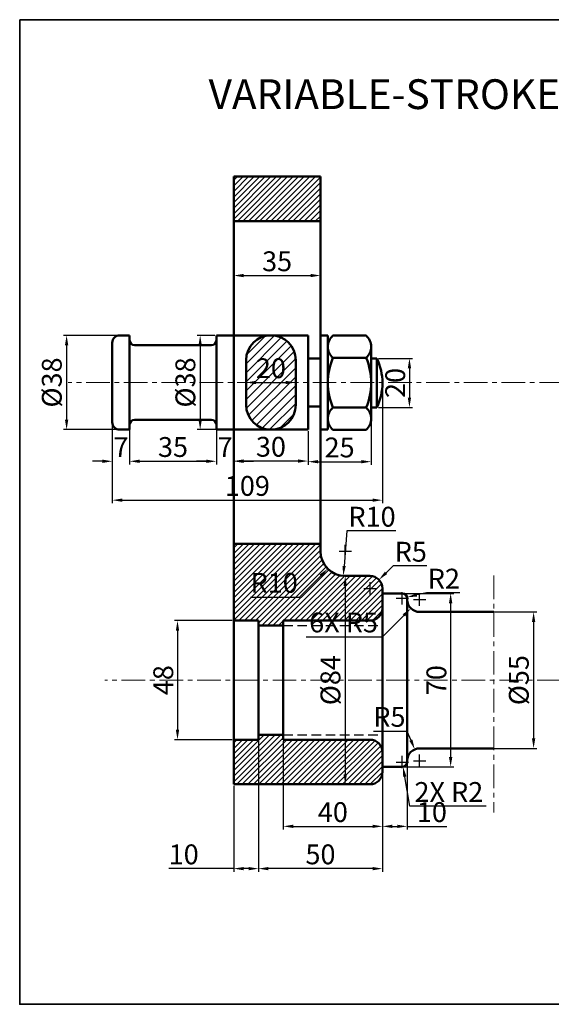
# Model space of a CAD drawing. Units: millimetres. Extents: x -135 to 382, y -21 to 376.
# Tile 1 of 2: x -135 to 80, y -21 to 376. Entities that reach past the tile are written whole.
import ezdxf

# ---------------------------------------------------------------- set-up
doc = ezdxf.new("R2010")
doc.units = ezdxf.units.MM
doc.header["$LTSCALE"] = 0.3
doc.linetypes.add('CENTER', pattern=[50.8, 31.75, -6.35, 6.35, -6.35])
doc.linetypes.add('DASHED', pattern=[19.05, 12.7, -6.35])
for name, color, linetype, lineweight in [('M-CNTR', 1, 'CENTER', 18), ('M-DIMS', 2, 'Continuous', 25), ('M-HATC', 8, 'Continuous', 18), ('M-HIDN', 6, 'DASHED', 25), ('M-OUTL', 7, 'Continuous', 50), ('M-TEXT', 3, 'Continuous', 25), ('M-TTLB', 7, 'Continuous', 35)]:
    doc.layers.add(name, color=color, linetype=linetype, lineweight=lineweight)
doc.styles.get("Standard").update_dxf_attribs({"font": 'arial.ttf'})
doc.dimstyles.new('ISO-25', dxfattribs={"dimtxt": 8, "dimasz": 4, "dimexe": 1.25, "dimexo": 0.625, "dimtad": 1, "dimtoh": 1, "dimdec": 0, "dimtxsty": 'Standard', "dimcen": 2.5, "dimadec": 0, "dimazin": 0, "dimtfac": 1, "dimtdec": 0, "dimtofl": 0, "dimtmove": 0, "dimatfit": 3, "dimfxl": 1, "dimarcsym": 0})

# ---------------------------------------------------------------- blocks, each defined once
blk = doc.blocks.new('*D1')
at = {"layer": 'Defpoints', "color": 0, "ltscale": 0.3, "transparency": 16777216}
for p in [(-48.44, 133.27), (-71.12, 85.27), (-48.44, 85.27)]:
    blk.add_point(p, dxfattribs=at)
at = {"layer": 'M-DIMS', "color": 0, "lineweight": -2, "ltscale": 0.3, "transparency": 16777216}
for p, q in [((-49.07, 133.27), (-72.37, 133.27)), ((-71.12, 129.27), (-71.12, 89.27)), ((-49.07, 85.27), (-72.37, 85.27))]:
    blk.add_line(p, q, dxfattribs=at)
at = {"layer": 'M-DIMS', "color": 0, "ltscale": 0.3, "transparency": 16777216}
for points in [[(-71.79, 129.27), (-70.46, 129.27), (-71.12, 133.27)], [(-71.79, 89.27), (-70.46, 89.27), (-71.12, 85.27)]]:
    blk.add_solid(points, dxfattribs=at)
at = {"layer": 'M-DIMS', "color": 0, "ltscale": 0.3, "transparency": 16777216, "insert": (-75.83, 109.27), "char_height": 8, "attachment_point": 5, "rotation": 90}
blk.add_mtext('48', dxfattribs=at)
blk = doc.blocks.new('*D2')
at = {"layer": 'Defpoints', "color": 0, "ltscale": 0.3, "transparency": 16777216}
for p in [(-3.44, 151.27), (-3.44, 67.27), (-3.44, 67.27)]:
    blk.add_point(p, dxfattribs=at)
at = {"layer": 'M-DIMS', "color": 0, "lineweight": -2, "ltscale": 0.3, "transparency": 16777216}
for p, q in [((-4.07, 151.27), (-4.69, 151.27)), ((-3.44, 147.27), (-3.44, 71.27)), ((-4.07, 67.27), (-4.69, 67.27))]:
    blk.add_line(p, q, dxfattribs=at)
at = {"layer": 'M-DIMS', "color": 0, "ltscale": 0.3, "transparency": 16777216}
for points in [[(-4.11, 147.27), (-2.78, 147.27), (-3.44, 151.27)], [(-4.11, 71.27), (-2.78, 71.27), (-3.44, 67.27)]]:
    blk.add_solid(points, dxfattribs=at)
at = {"layer": 'M-DIMS', "color": 0, "ltscale": 0.3, "transparency": 16777216, "insert": (-8.38, 109.27), "char_height": 8, "attachment_point": 5, "rotation": 90}
blk.add_mtext('%%C84', dxfattribs=at)
blk = doc.blocks.new('*D3')
at = {"layer": 'Defpoints', "color": 0, "ltscale": 0.3, "transparency": 16777216}
for p in [(15.56, 144.27), (15.56, 74.27), (39.08, 74.27)]:
    blk.add_point(p, dxfattribs=at)
at = {"layer": 'M-DIMS', "color": 0, "lineweight": -2, "ltscale": 0.3, "transparency": 16777216}
for p, q in [((16.18, 144.27), (40.33, 144.27)), ((39.08, 140.27), (39.08, 78.27)), ((16.18, 74.27), (40.33, 74.27))]:
    blk.add_line(p, q, dxfattribs=at)
at = {"layer": 'M-DIMS', "color": 0, "ltscale": 0.3, "transparency": 16777216}
for points in [[(38.41, 140.27), (39.75, 140.27), (39.08, 144.27)], [(38.41, 78.27), (39.75, 78.27), (39.08, 74.27)]]:
    blk.add_solid(points, dxfattribs=at)
at = {"layer": 'M-DIMS', "color": 0, "ltscale": 0.3, "transparency": 16777216, "insert": (34.37, 109.27), "char_height": 8, "attachment_point": 5, "rotation": 90}
blk.add_mtext('70', dxfattribs=at)
blk = doc.blocks.new('*D4')
at = {"layer": 'Defpoints', "color": 0, "ltscale": 0.3, "transparency": 16777216}
for p in [(49.48, 136.77), (49.48, 81.77), (72.56, 81.77)]:
    blk.add_point(p, dxfattribs=at)
at = {"layer": 'M-DIMS', "color": 0, "lineweight": -2, "ltscale": 0.3, "transparency": 16777216}
for p, q in [((50.1, 136.77), (73.81, 136.77)), ((72.56, 132.77), (72.56, 85.77)), ((50.1, 81.77), (73.81, 81.77))]:
    blk.add_line(p, q, dxfattribs=at)
at = {"layer": 'M-DIMS', "color": 0, "ltscale": 0.3, "transparency": 16777216}
for points in [[(71.89, 132.77), (73.22, 132.77), (72.56, 136.77)], [(71.89, 85.77), (73.22, 85.77), (72.56, 81.77)]]:
    blk.add_solid(points, dxfattribs=at)
at = {"layer": 'M-DIMS', "color": 0, "ltscale": 0.3, "transparency": 16777216, "insert": (67.62, 109.27), "char_height": 8, "attachment_point": 5, "rotation": 90}
blk.add_mtext('%%C55', dxfattribs=at)
blk = doc.blocks.new('*D5')
at = {"layer": 'Defpoints', "color": 0, "ltscale": 0.3, "transparency": 16777216}
for p in [(-38.44, 85.27), (-48.44, 67.27), (-38.44, 33.29)]:
    blk.add_point(p, dxfattribs=at)
at = {"layer": 'M-DIMS', "color": 0, "lineweight": -2, "ltscale": 0.3, "transparency": 16777216}
for p, q in [((-38.44, 84.64), (-38.44, 32.04)), ((-48.44, 66.64), (-48.44, 32.04)), ((-48.44, 33.29), (-74.58, 33.29)), ((-42.44, 33.29), (-44.44, 33.29))]:
    blk.add_line(p, q, dxfattribs=at)
at = {"layer": 'M-DIMS', "color": 0, "ltscale": 0.3, "transparency": 16777216}
for points in [[(-44.44, 33.95), (-44.44, 32.62), (-48.44, 33.29)], [(-42.44, 33.95), (-42.44, 32.62), (-38.44, 33.29)]]:
    blk.add_solid(points, dxfattribs=at)
at = {"layer": 'M-DIMS', "color": 0, "ltscale": 0.3, "transparency": 16777216, "insert": (-68.62, 38), "char_height": 8, "attachment_point": 5}
blk.add_mtext('10', dxfattribs=at)
blk = doc.blocks.new('*D6')
at = {"layer": 'Defpoints', "color": 0, "ltscale": 0.3, "transparency": 16777216}
for p in [(11.56, 74.27), (-38.44, 63.99), (-38.44, 33.29)]:
    blk.add_point(p, dxfattribs=at)
at = {"layer": 'M-DIMS', "color": 0, "lineweight": -2, "ltscale": 0.3, "transparency": 16777216}
for p, q in [((11.56, 73.64), (11.56, 32.04)), ((-38.44, 63.36), (-38.44, 32.04)), ((7.56, 33.29), (-34.44, 33.29))]:
    blk.add_line(p, q, dxfattribs=at)
at = {"layer": 'M-DIMS', "color": 0, "ltscale": 0.3, "transparency": 16777216}
for points in [[(-34.44, 33.95), (-34.44, 32.62), (-38.44, 33.29)], [(7.56, 33.95), (7.56, 32.62), (11.56, 33.29)]]:
    blk.add_solid(points, dxfattribs=at)
at = {"layer": 'M-DIMS', "color": 0, "ltscale": 0.3, "transparency": 16777216, "insert": (-13.44, 38), "char_height": 8, "attachment_point": 5}
blk.add_mtext('50', dxfattribs=at)
blk = doc.blocks.new('*D7')
at = {"layer": 'Defpoints', "color": 0, "ltscale": 0.3, "transparency": 16777216}
for p in [(-28.44, 85.27), (11.56, 85.27), (11.56, 50.33)]:
    blk.add_point(p, dxfattribs=at)
at = {"layer": 'M-DIMS', "color": 0, "lineweight": -2, "ltscale": 0.3, "transparency": 16777216}
for p, q in [((-28.44, 84.64), (-28.44, 49.08)), ((11.56, 84.64), (11.56, 49.08)), ((-24.44, 50.33), (7.56, 50.33))]:
    blk.add_line(p, q, dxfattribs=at)
at = {"layer": 'M-DIMS', "color": 0, "ltscale": 0.3, "transparency": 16777216}
for points in [[(-24.44, 51), (-24.44, 49.67), (-28.44, 50.33)], [(7.56, 51), (7.56, 49.67), (11.56, 50.33)]]:
    blk.add_solid(points, dxfattribs=at)
at = {"layer": 'M-DIMS', "color": 0, "ltscale": 0.3, "transparency": 16777216, "insert": (-8.44, 55.04), "char_height": 8, "attachment_point": 5}
blk.add_mtext('40', dxfattribs=at)
blk = doc.blocks.new('*D8')
at = {"layer": 'Defpoints', "color": 0, "ltscale": 0.3, "transparency": 16777216}
for p in [(11.56, 80.27), (21.56, 80.27), (21.56, 50.33)]:
    blk.add_point(p, dxfattribs=at)
at = {"layer": 'M-DIMS', "color": 0, "lineweight": -2, "ltscale": 0.3, "transparency": 16777216}
for p, q in [((11.56, 79.64), (11.56, 49.08)), ((21.56, 79.64), (21.56, 49.08)), ((15.56, 50.33), (17.56, 50.33)), ((21.56, 50.33), (37.49, 50.33))]:
    blk.add_line(p, q, dxfattribs=at)
at = {"layer": 'M-DIMS', "color": 0, "ltscale": 0.3, "transparency": 16777216}
for points in [[(15.56, 51), (15.56, 49.67), (11.56, 50.33)], [(17.56, 51), (17.56, 49.67), (21.56, 50.33)]]:
    blk.add_solid(points, dxfattribs=at)
at = {"layer": 'M-DIMS', "color": 0, "ltscale": 0.3, "transparency": 16777216, "insert": (31.52, 55.04), "char_height": 8, "attachment_point": 5}
blk.add_mtext('10', dxfattribs=at)
blk = doc.blocks.new('*D9')
at = {"layer": 'Defpoints', "color": 0, "ltscale": 0.3, "transparency": 16777216}
for p in [(-3.44, 161.27), (-4.22, 151.3)]:
    blk.add_point(p, dxfattribs=at)
at = {"layer": 'M-DIMS', "color": 0, "lineweight": -2, "ltscale": 0.3, "transparency": 16777216}
for p, q in [((-2.81, 169.41), (-3.91, 155.28)), ((16.91, 169.41), (-2.81, 169.41))]:
    blk.add_line(p, q, dxfattribs=at)
at = {"layer": 'M-DIMS', "color": 0, "ltscale": 0.3, "transparency": 16777216}
blk.add_solid([(-4.57, 155.34), (-3.25, 155.23), (-4.22, 151.3)], dxfattribs=at)
at = {"layer": 'M-DIMS', "color": 0, "ltscale": 0.3, "transparency": 16777216, "insert": (7.36, 174.12), "char_height": 8, "attachment_point": 5}
blk.add_mtext('R10', dxfattribs=at)
blk = doc.blocks.new('*D10')
at = {"layer": 'Defpoints', "color": 0, "ltscale": 0.3, "transparency": 16777216}
for p in [(10.15, 149.75), (6.56, 146.27)]:
    blk.add_point(p, dxfattribs=at)
at = {"layer": 'M-DIMS', "color": 0, "lineweight": -2, "ltscale": 0.3, "transparency": 16777216}
for p, q in [((15.9, 155.31), (13.02, 152.53)), ((29.48, 155.31), (15.9, 155.31)), ((6.56, 143.77), (6.56, 148.77)), ((4.06, 146.27), (9.06, 146.27))]:
    blk.add_line(p, q, dxfattribs=at)
at = {"layer": 'M-DIMS', "color": 0, "ltscale": 0.3, "transparency": 16777216}
blk.add_solid([(12.56, 153.01), (13.49, 152.05), (10.15, 149.75)], dxfattribs=at)
at = {"layer": 'M-DIMS', "color": 0, "ltscale": 0.3, "transparency": 16777216, "insert": (23, 160), "char_height": 8, "attachment_point": 5}
blk.add_mtext('R5', dxfattribs=at)
blk = doc.blocks.new('*D11')
at = {"layer": 'Defpoints', "color": 0, "ltscale": 0.3, "transparency": 16777216}
for p in [(19.56, 142.27), (21.51, 142.71)]:
    blk.add_point(p, dxfattribs=at)
at = {"layer": 'M-DIMS', "color": 0, "lineweight": -2, "ltscale": 0.3, "transparency": 16777216}
for p, q in [((19.56, 139.77), (19.56, 144.77)), ((29.3, 144.51), (25.4, 143.61)), ((42.75, 144.51), (29.3, 144.51)), ((17.06, 142.27), (22.06, 142.27))]:
    blk.add_line(p, q, dxfattribs=at)
at = {"layer": 'M-DIMS', "color": 0, "ltscale": 0.3, "transparency": 16777216}
blk.add_solid([(25.25, 144.26), (25.55, 142.96), (21.51, 142.71)], dxfattribs=at)
at = {"layer": 'M-DIMS', "color": 0, "ltscale": 0.3, "transparency": 16777216, "insert": (36.34, 149.15), "char_height": 8, "attachment_point": 5}
blk.add_mtext('R2', dxfattribs=at)
blk = doc.blocks.new('*D12')
at = {"layer": 'Defpoints', "color": 0, "ltscale": 0.3, "transparency": 16777216}
for p in [(24.6, 81.37), (26.56, 76.77)]:
    blk.add_point(p, dxfattribs=at)
at = {"layer": 'M-DIMS', "color": 0, "lineweight": -2, "ltscale": 0.3, "transparency": 16777216}
for p, q in [((7.89, 88.73), (21.47, 88.73)), ((21.47, 88.73), (23.04, 85.05)), ((24.06, 76.77), (29.06, 76.77)), ((26.56, 74.27), (26.56, 79.27))]:
    blk.add_line(p, q, dxfattribs=at)
at = {"layer": 'M-DIMS', "color": 0, "ltscale": 0.3, "transparency": 16777216}
blk.add_solid([(23.65, 85.31), (22.42, 84.79), (24.6, 81.37)], dxfattribs=at)
at = {"layer": 'M-DIMS', "color": 0, "ltscale": 0.3, "transparency": 16777216, "insert": (14.37, 93.43), "char_height": 8, "attachment_point": 5}
blk.add_mtext('R5', dxfattribs=at)
blk = doc.blocks.new('*D13')
at = {"layer": 'Defpoints', "color": 0, "ltscale": 0.3, "transparency": 16777216}
for p in [(-92.44, 248.27), (-115.87, 210.27), (-92.44, 210.27)]:
    blk.add_point(p, dxfattribs=at)
at = {"layer": 'M-DIMS', "color": 0, "lineweight": -2, "ltscale": 0.3, "transparency": 16777216}
for p, q in [((-93.07, 248.27), (-117.12, 248.27)), ((-115.87, 244.27), (-115.87, 214.27)), ((-93.07, 210.27), (-117.12, 210.27))]:
    blk.add_line(p, q, dxfattribs=at)
at = {"layer": 'M-DIMS', "color": 0, "ltscale": 0.3, "transparency": 16777216}
for points in [[(-116.54, 244.27), (-115.2, 244.27), (-115.87, 248.27)], [(-116.54, 214.27), (-115.2, 214.27), (-115.87, 210.27)]]:
    blk.add_solid(points, dxfattribs=at)
at = {"layer": 'M-DIMS', "color": 0, "ltscale": 0.3, "transparency": 16777216, "insert": (-120.8, 229.27), "char_height": 8, "attachment_point": 5, "rotation": 90}
blk.add_mtext('%%C38', dxfattribs=at)
blk = doc.blocks.new('*D14')
at = {"layer": 'Defpoints', "color": 0, "ltscale": 0.3, "transparency": 16777216}
for p in [(-97.44, 219.54), (-90.44, 219.54), (-90.44, 197.51)]:
    blk.add_point(p, dxfattribs=at)
at = {"layer": 'M-DIMS', "color": 0, "lineweight": -2, "ltscale": 0.3, "transparency": 16777216}
for p, q in [((-97.44, 218.92), (-97.44, 196.26)), ((-90.44, 218.92), (-90.44, 196.26)), ((-101.44, 197.51), (-105.44, 197.51)), ((-86.44, 197.51), (-82.44, 197.51))]:
    blk.add_line(p, q, dxfattribs=at)
at = {"layer": 'M-DIMS', "color": 0, "ltscale": 0.3, "transparency": 16777216}
for points in [[(-101.44, 198.17), (-101.44, 196.84), (-97.44, 197.51)], [(-86.44, 198.17), (-86.44, 196.84), (-90.44, 197.51)]]:
    blk.add_solid(points, dxfattribs=at)
at = {"layer": 'M-DIMS', "color": 0, "ltscale": 0.3, "transparency": 16777216, "insert": (-93.94, 202.13), "char_height": 8, "attachment_point": 5}
blk.add_mtext('7', dxfattribs=at)
blk = doc.blocks.new('*D15')
at = {"layer": 'Defpoints', "color": 0, "ltscale": 0.3, "transparency": 16777216}
for p in [(-90.44, 222.54), (-55.44, 222.54), (-55.44, 197.51)]:
    blk.add_point(p, dxfattribs=at)
at = {"layer": 'M-DIMS', "color": 0, "lineweight": -2, "ltscale": 0.3, "transparency": 16777216}
for p, q in [((-90.44, 221.92), (-90.44, 196.26)), ((-55.44, 221.92), (-55.44, 196.26)), ((-86.44, 197.51), (-59.44, 197.51))]:
    blk.add_line(p, q, dxfattribs=at)
at = {"layer": 'M-DIMS', "color": 0, "ltscale": 0.3, "transparency": 16777216}
for points in [[(-86.44, 198.17), (-86.44, 196.84), (-90.44, 197.51)], [(-59.44, 198.17), (-59.44, 196.84), (-55.44, 197.51)]]:
    blk.add_solid(points, dxfattribs=at)
at = {"layer": 'M-DIMS', "color": 0, "ltscale": 0.3, "transparency": 16777216, "insert": (-72.94, 202.22), "char_height": 8, "attachment_point": 5}
blk.add_mtext('35', dxfattribs=at)
blk = doc.blocks.new('*D16')
at = {"layer": 'Defpoints', "color": 0, "ltscale": 0.3, "transparency": 16777216}
for p in [(-55.44, 222.54), (-48.44, 218.5), (-48.44, 197.51)]:
    blk.add_point(p, dxfattribs=at)
at = {"layer": 'M-DIMS', "color": 0, "lineweight": -2, "ltscale": 0.3, "transparency": 16777216}
for p, q in [((-55.44, 221.92), (-55.44, 196.26)), ((-48.44, 217.88), (-48.44, 196.26)), ((-59.44, 197.51), (-63.44, 197.51)), ((-44.44, 197.51), (-40.44, 197.51))]:
    blk.add_line(p, q, dxfattribs=at)
at = {"layer": 'M-DIMS', "color": 0, "ltscale": 0.3, "transparency": 16777216}
for points in [[(-59.44, 198.17), (-59.44, 196.84), (-55.44, 197.51)], [(-44.44, 198.17), (-44.44, 196.84), (-48.44, 197.51)]]:
    blk.add_solid(points, dxfattribs=at)
at = {"layer": 'M-DIMS', "color": 0, "ltscale": 0.3, "transparency": 16777216, "insert": (-51.94, 202.13), "char_height": 8, "attachment_point": 5}
blk.add_mtext('7', dxfattribs=at)
blk = doc.blocks.new('*D17')
at = {"layer": 'Defpoints', "color": 0, "ltscale": 0.3, "transparency": 16777216}
for p in [(-18.44, 210.27), (-48.44, 201.14), (-48.44, 197.6)]:
    blk.add_point(p, dxfattribs=at)
at = {"layer": 'M-DIMS', "color": 0, "lineweight": -2, "ltscale": 0.3, "transparency": 16777216}
for p, q in [((-18.44, 209.64), (-18.44, 196.35)), ((-48.44, 200.52), (-48.44, 196.35)), ((-22.44, 197.6), (-44.44, 197.6))]:
    blk.add_line(p, q, dxfattribs=at)
at = {"layer": 'M-DIMS', "color": 0, "ltscale": 0.3, "transparency": 16777216}
for points in [[(-44.44, 198.27), (-44.44, 196.94), (-48.44, 197.6)], [(-22.44, 198.27), (-22.44, 196.94), (-18.44, 197.6)]]:
    blk.add_solid(points, dxfattribs=at)
at = {"layer": 'M-DIMS', "color": 0, "ltscale": 0.3, "transparency": 16777216, "insert": (-33.44, 202.32), "char_height": 8, "attachment_point": 5}
blk.add_mtext('30', dxfattribs=at)
blk = doc.blocks.new('*D18')
at = {"layer": 'Defpoints', "color": 0, "ltscale": 0.3, "transparency": 16777216}
for p in [(-97.44, 229.27), (11.56, 229.27), (11.56, 181.83)]:
    blk.add_point(p, dxfattribs=at)
at = {"layer": 'M-DIMS', "color": 0, "lineweight": -2, "ltscale": 0.3, "transparency": 16777216}
for p, q in [((-97.44, 228.64), (-97.44, 180.58)), ((11.56, 228.64), (11.56, 180.58)), ((-93.44, 181.83), (7.56, 181.83))]:
    blk.add_line(p, q, dxfattribs=at)
at = {"layer": 'M-DIMS', "color": 0, "ltscale": 0.3, "transparency": 16777216}
for points in [[(-93.44, 182.5), (-93.44, 181.17), (-97.44, 181.83)], [(7.56, 182.5), (7.56, 181.17), (11.56, 181.83)]]:
    blk.add_solid(points, dxfattribs=at)
at = {"layer": 'M-DIMS', "color": 0, "ltscale": 0.3, "transparency": 16777216, "insert": (-42.94, 186.54), "char_height": 8, "attachment_point": 5}
blk.add_mtext('109', dxfattribs=at)
blk = doc.blocks.new('*D19')
at = {"layer": 'Defpoints', "color": 0, "ltscale": 0.3, "transparency": 16777216}
for p in [(7.01, 214.74), (-18.44, 203), (7.01, 197.34)]:
    blk.add_point(p, dxfattribs=at)
at = {"layer": 'M-DIMS', "color": 0, "lineweight": -2, "ltscale": 0.3, "transparency": 16777216}
for p, q in [((7.01, 214.11), (7.01, 196.09)), ((-18.44, 202.37), (-18.44, 196.09)), ((-14.44, 197.34), (3.01, 197.34))]:
    blk.add_line(p, q, dxfattribs=at)
at = {"layer": 'M-DIMS', "color": 0, "ltscale": 0.3, "transparency": 16777216}
for points in [[(-14.44, 198.01), (-14.44, 196.68), (-18.44, 197.34)], [(3.01, 198.01), (3.01, 196.68), (7.01, 197.34)]]:
    blk.add_solid(points, dxfattribs=at)
at = {"layer": 'M-DIMS', "color": 0, "ltscale": 0.3, "transparency": 16777216, "insert": (-5.72, 202.05), "char_height": 8, "attachment_point": 5}
blk.add_mtext('25', dxfattribs=at)
blk = doc.blocks.new('*D20')
at = {"layer": 'Defpoints', "color": 0, "ltscale": 0.3, "transparency": 16777216}
for p in [(-13.44, 272.39), (-48.44, 268.37), (-13.44, 268.37)]:
    blk.add_point(p, dxfattribs=at)
at = {"layer": 'M-DIMS', "color": 0, "lineweight": -2, "ltscale": 0.3, "transparency": 16777216}
for p, q in [((-48.44, 269), (-48.44, 273.64)), ((-44.44, 272.39), (-17.44, 272.39)), ((-13.44, 269), (-13.44, 273.64))]:
    blk.add_line(p, q, dxfattribs=at)
at = {"layer": 'M-DIMS', "color": 0, "ltscale": 0.3, "transparency": 16777216}
for points in [[(-44.44, 273.05), (-44.44, 271.72), (-48.44, 272.39)], [(-17.44, 273.05), (-17.44, 271.72), (-13.44, 272.39)]]:
    blk.add_solid(points, dxfattribs=at)
at = {"layer": 'M-DIMS', "color": 0, "ltscale": 0.3, "transparency": 16777216, "insert": (-30.94, 277.1), "char_height": 8, "attachment_point": 5}
blk.add_mtext('35', dxfattribs=at)
blk = doc.blocks.new('*D21')
at = {"layer": 'Defpoints', "color": 0, "ltscale": 0.3, "transparency": 16777216}
for p in [(-55.44, 248.27), (-61.98, 210.27), (-54.29, 210.27)]:
    blk.add_point(p, dxfattribs=at)
at = {"layer": 'M-DIMS', "color": 0, "lineweight": -2, "ltscale": 0.3, "transparency": 16777216}
for p, q in [((-56.07, 248.27), (-63.23, 248.27)), ((-61.98, 244.27), (-61.98, 214.27)), ((-54.91, 210.27), (-63.23, 210.27))]:
    blk.add_line(p, q, dxfattribs=at)
at = {"layer": 'M-DIMS', "color": 0, "ltscale": 0.3, "transparency": 16777216}
for points in [[(-62.65, 244.27), (-61.31, 244.27), (-61.98, 248.27)], [(-62.65, 214.27), (-61.31, 214.27), (-61.98, 210.27)]]:
    blk.add_solid(points, dxfattribs=at)
at = {"layer": 'M-DIMS', "color": 0, "ltscale": 0.3, "transparency": 16777216, "insert": (-66.91, 229.27), "char_height": 8, "attachment_point": 5, "rotation": 90}
blk.add_mtext('%%C38', dxfattribs=at)
blk = doc.blocks.new('*D22')
at = {"layer": 'Defpoints', "color": 0, "ltscale": 0.3, "transparency": 16777216}
for p in [(9.28, 239), (9.28, 219.16), (22.45, 219.16)]:
    blk.add_point(p, dxfattribs=at)
at = {"layer": 'M-DIMS', "color": 0, "lineweight": -2, "ltscale": 0.3, "transparency": 16777216}
for p, q in [((9.91, 239), (23.7, 239)), ((22.45, 235), (22.45, 223.16)), ((9.91, 219.16), (23.7, 219.16))]:
    blk.add_line(p, q, dxfattribs=at)
at = {"layer": 'M-DIMS', "color": 0, "ltscale": 0.3, "transparency": 16777216}
for points in [[(21.79, 235), (23.12, 235), (22.45, 239)], [(21.79, 223.16), (23.12, 223.16), (22.45, 219.16)]]:
    blk.add_solid(points, dxfattribs=at)
at = {"layer": 'M-DIMS', "color": 0, "ltscale": 0.3, "transparency": 16777216, "insert": (17.75, 229.08), "char_height": 8, "attachment_point": 5, "rotation": 90}
blk.add_mtext('20', dxfattribs=at)
blk = doc.blocks.new('*D23')
at = {"layer": 'Defpoints', "color": 0, "ltscale": 0.3, "transparency": 16777216}
for p in [(-43.44, 229.27), (-23.44, 229.27), (-23.44, 229.27)]:
    blk.add_point(p, dxfattribs=at)
at = {"layer": 'M-DIMS', "color": 0, "lineweight": -2, "ltscale": 0.3, "transparency": 16777216}
for p, q in [((-43.44, 229.89), (-43.44, 230.52)), ((-23.44, 229.89), (-23.44, 230.52)), ((-39.44, 229.27), (-27.44, 229.27))]:
    blk.add_line(p, q, dxfattribs=at)
at = {"layer": 'M-DIMS', "color": 0, "ltscale": 0.3, "transparency": 16777216}
for points in [[(-39.44, 229.93), (-39.44, 228.6), (-43.44, 229.27)], [(-27.44, 229.93), (-27.44, 228.6), (-23.44, 229.27)]]:
    blk.add_solid(points, dxfattribs=at)
at = {"layer": 'M-DIMS', "color": 0, "ltscale": 0.3, "transparency": 16777216, "insert": (-33.44, 233.98), "char_height": 8, "attachment_point": 5}
blk.add_mtext('20', dxfattribs=at)
blk = doc.blocks.new('*D37')
at = {"layer": 'Defpoints', "color": 0, "ltscale": 0.3, "transparency": 16777216}
for p in [(-3.44, 161.27), (-10.51, 154.2)]:
    blk.add_point(p, dxfattribs=at)
at = {"layer": 'M-DIMS', "color": 0, "lineweight": -2, "ltscale": 0.3, "transparency": 16777216}
for p, q in [((-3.44, 158.77), (-3.44, 163.77)), ((-5.94, 161.27), (-0.94, 161.27)), ((-21.95, 142.76), (-13.34, 151.37)), ((-41.66, 142.76), (-21.95, 142.76))]:
    blk.add_line(p, q, dxfattribs=at)
at = {"layer": 'M-DIMS', "color": 0, "ltscale": 0.3, "transparency": 16777216}
blk.add_solid([(-13.81, 151.84), (-12.87, 150.9), (-10.51, 154.2)], dxfattribs=at)
at = {"layer": 'M-DIMS', "color": 0, "ltscale": 0.3, "transparency": 16777216, "insert": (-32.12, 147.47), "char_height": 8, "attachment_point": 5}
blk.add_mtext('R10', dxfattribs=at)
blk = doc.blocks.new('*D38')
at = {"layer": 'Defpoints', "color": 0, "ltscale": 0.3, "transparency": 16777216}
for p in [(26.56, 141.77), (23.03, 138.23)]:
    blk.add_point(p, dxfattribs=at)
at = {"layer": 'M-DIMS', "color": 0, "lineweight": -2, "ltscale": 0.3, "transparency": 16777216}
for p, q in [((26.56, 139.27), (26.56, 144.27)), ((24.06, 141.77), (29.06, 141.77)), ((11.61, 126.78), (20.2, 135.39)), ((-19.21, 126.78), (11.61, 126.78))]:
    blk.add_line(p, q, dxfattribs=at)
at = {"layer": 'M-DIMS', "color": 0, "ltscale": 0.3, "transparency": 16777216}
blk.add_solid([(19.73, 135.86), (20.67, 134.92), (23.03, 138.23)], dxfattribs=at)
at = {"layer": 'M-DIMS', "color": 0, "ltscale": 0.3, "transparency": 16777216, "insert": (-4.11, 131.49), "char_height": 8, "attachment_point": 5}
blk.add_mtext('6X R5', dxfattribs=at)
blk = doc.blocks.new('*D39')
at = {"layer": 'Defpoints', "color": 0, "ltscale": 0.3, "transparency": 16777216}
for p in [(19.56, 76.27), (19.9, 74.3)]:
    blk.add_point(p, dxfattribs=at)
at = {"layer": 'M-DIMS', "color": 0, "lineweight": -2, "ltscale": 0.3, "transparency": 16777216}
for p, q in [((17.06, 76.27), (22.06, 76.27)), ((19.56, 73.77), (19.56, 78.77)), ((22.66, 58.5), (20.59, 70.36)), ((53.43, 58.5), (22.66, 58.5))]:
    blk.add_line(p, q, dxfattribs=at)
at = {"layer": 'M-DIMS', "color": 0, "ltscale": 0.3, "transparency": 16777216}
blk.add_solid([(21.25, 70.47), (19.93, 70.24), (19.9, 74.3)], dxfattribs=at)
at = {"layer": 'M-DIMS', "color": 0, "ltscale": 0.3, "transparency": 16777216, "insert": (38.36, 63.14), "char_height": 8, "attachment_point": 5}
blk.add_mtext('2X R2', dxfattribs=at)

msp = doc.modelspace()

# ---------------------------------------------------------------- hatches: boundary and pattern name
at = {"layer": 'M-HATC', "ltscale": 0.3}
h = msp.add_hatch(dxfattribs=at)
h.set_pattern_fill('ANSI31', color=256, scale=0.5)
h.paths.add_polyline_path([(-13.44, 312.27), (-48.44, 312.27), (-48.44, 294.27), (-13.44, 294.27)])
h.paths.add_polyline_path([(11.56, 146.27, 0.414214), (6.56, 151.27), (-3.44, 151.27, -0.414214), (-13.44, 161.27), (-13.44, 164.27), (-48.44, 164.27), (-48.44, 133.27), (-38.44, 133.27), (-38.44, 131.27), (-28.44, 131.27), (-28.44, 133.27), (6.56, 133.27, 0.414214), (11.56, 138.27)])
h.paths.add_polyline_path([(11.56, 80.27, 0.414214), (6.56, 85.27), (-28.44, 85.27), (-28.44, 87.27), (-38.44, 87.27), (-38.44, 85.27), (-48.44, 85.27), (-48.44, 67.27), (6.56, 67.27, 0.414214), (11.56, 72.27)])
h = msp.add_hatch(dxfattribs=at)
h.set_pattern_fill('ANSI31', color=256, scale=0.8)
h.paths.add_polyline_path([(-23.44, 238.27, 1), (-43.44, 238.27), (-43.44, 229.27), (-23.44, 229.27)])
h.paths.add_polyline_path([(-23.44, 229.27), (-43.44, 229.27), (-43.44, 220.27, 1), (-23.44, 220.27)])

# ---------------------------------------------------------------- linework, layer by layer
at = {"layer": 'M-CNTR'}
for p, q in [((145.36, 229.27), (-115.25, 229.27)), ((56.56, 151.5), (56.56, 55.89)), ((266.38, 109.27), (-100.48, 109.27))]:
    msp.add_line(p, q, dxfattribs=at)
at = {"layer": 'M-HIDN'}
for p, q in [((-28.44, 131.27), (11.56, 131.27)), ((-28.44, 87.27), (11.56, 87.27))]:
    msp.add_line(p, q, dxfattribs=at)
at = {"layer": 'M-OUTL'}
for p, q in [((-48.44, 312.27), (-48.44, 67.27)), ((-48.44, 312.27), (-13.44, 312.27)), ((-13.44, 312.27), (-13.44, 161.27)), ((6.56, 151.27), (-3.44, 151.27)), ((11.56, 72.27), (11.56, 146.27)), ((11.56, 144.27), (19.56, 144.27)), ((21.56, 142.27), (21.56, 141.77)), ((21.56, 76.27), (21.56, 142.27)), ((26.56, 136.77), (56.56, 136.77)), ((-48.44, 133.27), (-48.44, 85.27)), ((-38.44, 133.27), (-48.44, 133.27)), ((-38.44, 85.27), (-38.44, 133.27)), ((-38.44, 131.27), (-38.44, 87.27)), ((-38.44, 131.27), (-28.44, 131.27)), ((6.56, 133.27), (-28.44, 133.27)), ((-28.44, 133.27), (-28.44, 85.27)), ((-28.44, 87.27), (-28.44, 131.27)), ((-48.44, 85.27), (-38.44, 85.27)), ((-38.44, 87.27), (-28.44, 87.27)), ((-28.44, 85.27), (6.56, 85.27)), ((56.56, 81.77), (26.56, 81.77)), ((21.56, 76.77), (21.56, 76.27)), ((19.56, 74.27), (11.56, 74.27)), ((-48.44, 67.27), (6.56, 67.27))]:
    msp.add_line(p, q, dxfattribs=at)
at = {"layer": 'M-OUTL', "ltscale": 0.3}
for p, q in [((-13.44, 294.27), (-48.44, 294.27)), ((-94.44, 248.27), (-90.44, 248.27)), ((-90.44, 248.27), (-90.44, 246.27)), ((-90.44, 246.27), (-90.44, 210.27)), ((-55.44, 246.27), (-55.44, 248.27)), ((-55.44, 248.27), (-48.44, 248.27)), ((-55.44, 246.27), (-55.44, 212.27)), ((-48.44, 248.27), (-48.44, 210.27)), ((-48.44, 248.27), (-18.44, 248.27)), ((-18.44, 248.27), (-18.44, 210.27)), ((-13.44, 248.27), (-10.44, 248.27)), ((-10.44, 248.27), (-10.44, 210.27)), ((-1.41, 248.16), (-8.44, 248.16)), ((5.01, 248.16), (-1.41, 248.16)), ((-97.44, 213.27), (-97.44, 245.27)), ((-88.44, 244.27), (-57.44, 244.27)), ((-10.44, 243.95), (-10.44, 214.59)), ((7.01, 214.59), (7.01, 243.95)), ((-43.44, 220.27), (-43.44, 238.27)), ((-23.44, 220.27), (-23.44, 238.27)), ((-13.44, 239), (-18.44, 239)), ((-8.44, 239.16), (-1.41, 239.16)), ((-1.41, 239.16), (5.01, 239.16)), ((7.01, 239), (9.28, 239)), ((9.28, 239), (9.28, 219.16)), ((11.56, 229.08), (11.56, 229.27)), ((-13.44, 219.54), (-18.44, 219.54)), ((-8.44, 219.16), (-1.41, 219.16)), ((-1.41, 219.16), (5.01, 219.16)), ((7.01, 219.16), (9.28, 219.16)), ((-57.44, 214.27), (-88.44, 214.27)), ((-55.44, 210.27), (-55.44, 212.27)), ((-90.44, 210.27), (-94.44, 210.27)), ((-48.44, 210.27), (-55.44, 210.27)), ((-18.44, 210.27), (-48.44, 210.27)), ((-10.44, 210.27), (-13.44, 210.27)), ((-8.44, 210.16), (-1.41, 210.16)), ((-1.41, 210.16), (5.01, 210.16)), ((-48.44, 164.27), (-13.44, 164.27))]:
    msp.add_line(p, q, dxfattribs=at)
for centre, radius, start, end in [((-94.44, 245.27), 3, 90, 180), ((-88.44, 246.27), 2, 180, 270), ((-57.44, 246.27), 2, 270, 0), ((-33.44, 238.27), 10, 0, 180), ((-4.4, 243.66), 6.05, 131.9333, 228.0667), ((0.97, 243.66), 6.05, 311.9333, 48.0667), ((15.56, 229.16), 26, 157.3801, 202.6199), ((-18.99, 229.16), 26, 337.3801, 22.6199), ((-11.2, 229.08), 22.76, 334.1686, 25.8314), ((-33.44, 220.27), 10, 180, 0), ((-4.38, 214.66), 6.06, 132.0649, 227.9351), ((0.95, 214.66), 6.06, 312.0649, 47.9351), ((-94.44, 213.27), 3, 180, 270), ((-88.44, 212.27), 2, 90, 180), ((-57.44, 212.27), 2, 0, 90)]:
    msp.add_arc(centre, radius, start, end, dxfattribs=at)
at = {"layer": 'M-OUTL'}
for centre, radius, start, end in [((-3.44, 161.27), 10, 180, 270), ((6.56, 146.27), 5, 0, 90), ((19.56, 142.27), 2, 0, 90), ((26.56, 141.77), 5, 180, 270), ((6.56, 138.27), 5, 270, 0), ((6.56, 80.27), 5, 0, 90), ((26.56, 76.77), 5, 90, 180), ((19.56, 76.27), 2, 270, 0), ((6.56, 72.27), 5, 270, 0)]:
    msp.add_arc(centre, radius, start, end, dxfattribs=at)
at = {"layer": 'M-TTLB', "ltscale": 0.3}
msp.add_lwpolyline([(-134.8, 375.53), (381.64, 375.53), (381.64, -21.41), (-134.8, -21.41)], close=True, dxfattribs=at)

# ---------------------------------------------------------------- texts
at = {"layer": 'M-TEXT', "ltscale": 0.3, "insert": (-77.37, 351.5), "char_height": 12, "attachment_point": 1}
msp.add_mtext_dynamic_manual_height_columns('\\pxqc;VARIABLE-STROKE CRANK LEVER', width=287.9223, gutter_width=12.5, heights=[0], dxfattribs=at)

# ---------------------------------------------------------------- dimensions: what is measured, and where the dimension line sits
at = {"layer": 'M-DIMS', "ltscale": 0.3}
for base, p1, p2, picture, middle in [((-13.44, 272.39), (-48.44, 268.37), (-13.44, 268.37), '*D20', (-30.94, 277.1)), ((-23.44, 229.27), (-43.44, 229.27), (-23.44, 229.27), '*D23', (-33.44, 233.98)), ((11.56, 181.83), (-97.44, 229.27), (11.56, 229.27), '*D18', (-42.94, 186.54)), ((-55.44, 197.51), (-90.44, 222.54), (-55.44, 222.54), '*D15', (-72.94, 202.22)), ((-48.44, 197.51), (-55.44, 222.54), (-48.44, 218.5), '*D16', (-51.94, 202.13)), ((-90.44, 197.51), (-97.44, 219.54), (-90.44, 219.54), '*D14', (-93.94, 202.13)), ((7.01, 197.34), (-18.44, 203), (7.01, 214.74), '*D19', (-5.72, 202.05)), ((-48.44, 197.6), (-18.44, 210.27), (-48.44, 201.14), '*D17', (-33.44, 202.32)), ((11.56, 50.33), (-28.44, 85.27), (11.56, 85.27), '*D7', (-8.44, 55.04)), ((21.56, 50.33), (11.56, 80.27), (21.56, 80.27), '*D8', (31.52, 55.04))]:
    dim = msp.add_linear_dim(base=base, p1=p1, p2=p2, dimstyle='ISO-25', override={"dimclrd": 0, "dimclre": 0, "dimclrt": 0}, dxfattribs=at)
    dim.commit()
    dim.dimension.update_dxf_attribs({"geometry": picture, "text_midpoint": middle})
for base, p1, p2, picture, middle in [((-115.87, 210.27), (-92.44, 248.27), (-92.44, 210.27), '*D13', (-120.8, 229.27)), ((-61.98, 210.27), (-55.44, 248.27), (-54.29, 210.27), '*D21', (-66.91, 229.27)), ((-3.44, 67.27), (-3.44, 151.27), (-3.44, 67.27), '*D2', (-8.38, 109.27)), ((72.56, 81.77), (49.48, 136.77), (49.48, 81.77), '*D4', (67.62, 109.27))]:
    dim = msp.add_linear_dim(base=base, p1=p1, p2=p2, angle=90, text='%%C<>', dimstyle='ISO-25', override={"dimclrd": 0, "dimclre": 0, "dimclrt": 0}, dxfattribs=at)
    dim.commit()
    dim.dimension.update_dxf_attribs({"geometry": picture, "text_midpoint": middle})
for base, p1, p2, picture, middle in [((22.45, 219.16), (9.28, 239), (9.28, 219.16), '*D22', (17.75, 229.08)), ((39.08, 74.27), (15.56, 144.27), (15.56, 74.27), '*D3', (34.37, 109.27)), ((-71.12, 85.27), (-48.44, 133.27), (-48.44, 85.27), '*D1', (-75.83, 109.27))]:
    dim = msp.add_linear_dim(base=base, p1=p1, p2=p2, angle=90, dimstyle='ISO-25', override={"dimclrd": 0, "dimclre": 0, "dimclrt": 0}, dxfattribs=at)
    dim.commit()
    dim.dimension.update_dxf_attribs({"geometry": picture, "text_midpoint": middle})
dim = msp.add_radius_dim(center=(-3.44, 161.27), mpoint=(-4.22, 151.3), dimstyle='ISO-25', override={"dimclrd": 0, "dimclre": 0, "dimclrt": 0}, dxfattribs=at)
dim.commit()
dim.dimension.update_dxf_attribs({"geometry": '*D9', "text_midpoint": (7.36, 169.41), "dimtype": 164})
for center, mpoint, override, picture, middle in [((-3.44, 161.27), (-10.51, 154.2), {"dimdec": 0, "dimlfac": 1, "dimrnd": 0, "dimzin": 0, "dimdsep": 46, "dimlunit": 2}, '*D37', (-32.12, 147.47)), ((6.56, 146.27), (10.15, 149.75), {"dimclrd": 0, "dimclre": 0, "dimclrt": 0}, '*D10', (23, 160)), ((19.56, 142.27), (21.51, 142.71), {"dimclrd": 0, "dimclre": 0, "dimclrt": 0}, '*D11', (36.34, 149.15)), ((26.56, 76.77), (24.6, 81.37), {"dimclrd": 0, "dimclre": 0, "dimclrt": 0}, '*D12', (14.37, 93.43))]:
    dim = msp.add_radius_dim(center=center, mpoint=mpoint, dimstyle='ISO-25', override=override, dxfattribs=at)
    dim.commit()
    dim.dimension.update_dxf_attribs({"geometry": picture, "text_midpoint": middle})
for center, mpoint, text, picture, middle in [((26.56, 141.77), (23.03, 138.23), '6X <>', '*D38', (-4.11, 131.49)), ((19.56, 76.27), (19.9, 74.3), '2X <>', '*D39', (38.36, 63.14))]:
    dim = msp.add_radius_dim(center=center, mpoint=mpoint, text=text, dimstyle='ISO-25', override={"dimdec": 0, "dimlfac": 1, "dimrnd": 0, "dimzin": 0, "dimdsep": 46, "dimlunit": 2}, dxfattribs=at)
    dim.commit()
    dim.dimension.update_dxf_attribs({"geometry": picture, "text_midpoint": middle})
for p1, p2, picture, middle in [((-48.44, 67.27), (-38.44, 85.27), '*D5', (-68.62, 33.29)), ((11.56, 74.27), (-38.44, 63.99), '*D6', (-13.44, 33.29))]:
    dim = msp.add_linear_dim(base=(-38.44, 33.29), p1=p1, p2=p2, dimstyle='ISO-25', override={"dimclrd": 0, "dimclre": 0, "dimclrt": 0}, dxfattribs=at)
    dim.commit()
    dim.dimension.update_dxf_attribs({"geometry": picture, "text_midpoint": middle, "dimtype": 160})

doc.saveas('drawing.dxf')
